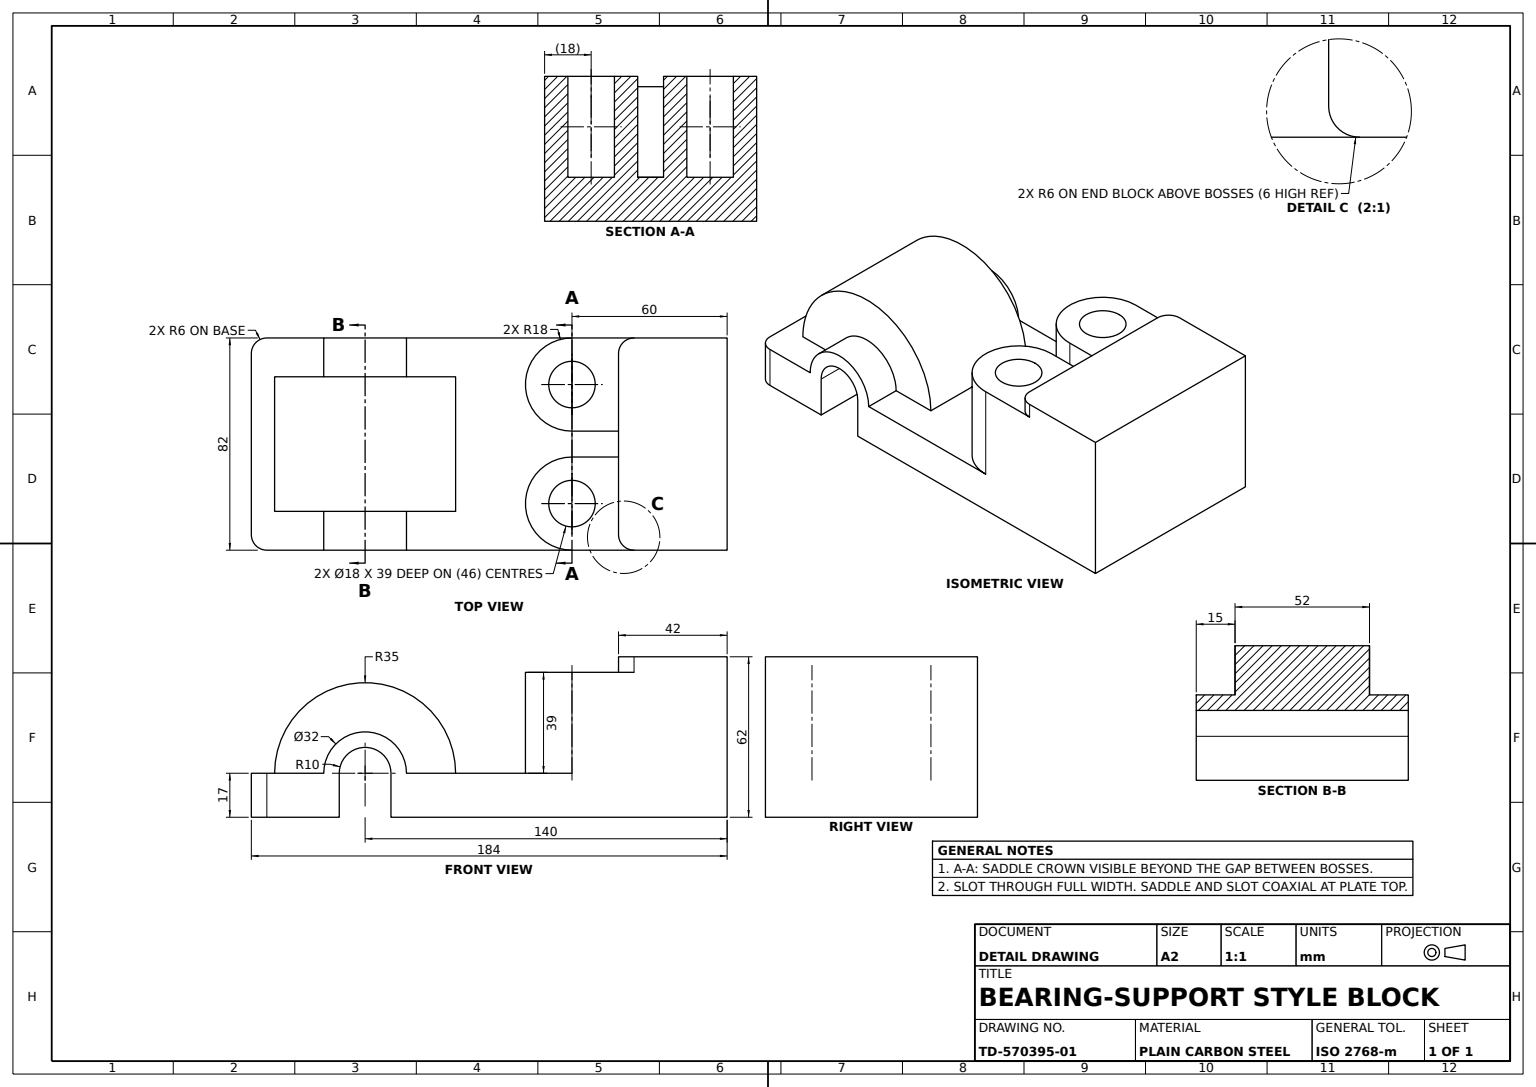
SolidWorks part; units mm, degrees
material "Plain Carbon Steel"
ref_plane "Front Plane" through (0, 0, 0) normal (0, 0, 1) x (1, 0, 0)
ref_plane "Top Plane" through (0, 0, 0) normal (0, 1, 0) x (1, 0, 0)
ref_plane "Right Plane" through (0, 0, 0) normal (1, 0, 0) x (0, 0, -1)
sketch "Base Plate Sketch" plane through (0, 0, 0) normal (0, 1, 0) x (1, 0, 0)
  line L1 (-86, -41) -> (92, -41)
  line L2 (-92, -35) -> (-92, 35)
  line L3 (-86, 41) -> (92, 41)
  line L4 (92, -41) -> (92, 41)
  line L5 (-92, -41) -> (92, 41) construction
  line L6 (-92, 41) -> (92, -41) construction
  arc A0 (-86, -41) -> (-92, -35) centre (-86, -35) cw
  arc A1 (-92, 35) -> (-86, 41) centre (-86, 35) cw
  point P0 (0, 0)
  dimension "D3" = 6
  dimension "D1" = 82
  dimension "D2" = 184
extrude "Base Plate 184x82x17" add sketch "Base Plate Sketch" along normal blind 17
sketch "Bearing Saddle Sketch" plane through (0, 17, 0) normal (0, 1, 0) x (1, 0, 0)
  line L0 (92, 41) -> (-86, 41) construction
  line L1 (92, -41) -> (56, -41)
  line L2 (92, -41) -> (92, 41)
  line L3 (92, 41) -> (56, 41)
  line L4 (50, -35) -> (50, 35)
  arc A0 (56, -41) -> (50, -35) centre (56, -35) cw
  arc A1 (56, 41) -> (50, 35) centre (56, 35) ccw
  point P11 (50, 41)
  dimension "D2" = 6
  dimension "D1" = 42
extrude "Bearing Saddle" add sketch "Bearing Saddle Sketch" along normal blind 45
sketch "Raised Pad Sketch" plane through (0, 0, 41) normal (0, 0, 1) x (1, 0, 0)
  line L0 (-86, 17) -> (56, 17) construction
  line L1 (92, 62) -> (92, 0) construction
  line L2 (-58, 17) -> (-58, 0)
  line L3 (-86, 0) -> (92, 0) construction
  line L4 (-58, 0) -> (-38, 0)
  line L5 (-38, 0) -> (-38, 17)
  arc A0 (-38, 17) -> (-58, 17) centre (-48, 17) ccw
  dimension "D1" = 140
  dimension "D2" = 10
extrude "Raised Pad" add sketch "Raised Pad Sketch" against normal blind 82
sketch "Step Profile Sketch" plane through (0, 0, 41) normal (0, 0, 1) x (1, 0, 0)
  line L0 (-58, 17) -> (-58, 0)
  line L1 (-86, 0) -> (92, 0) construction
  line L2 (-58, 0) -> (-38, 0)
  line L3 (-38, 0) -> (-38, 17)
  line L4 (-86, 17) -> (-64, 17)
  line L5 (-38, 17) -> (-32, 17)
  line L6 (-58, 17) -> (-64, 17)
  arc A0 (-58, 17) -> (-38, 17) centre (-48, 17) cw
  arc A1 (-32, 17) -> (-64, 17) centre (-48, 17) ccw
  line M5 (56, 17) -> (-38, 17)
  arc M6 (-38, 17) -> (-58, 17) centre (-48, 17) ccw
  line M7 (-58, 17) -> (-86, 17)
  dimension "D1" = 10
  dimension "D2" = 32
extrude "Step Profile" add sketch "Step Profile Sketch" against normal blind 82 contours A1 M5 M7 M6
sketch "Slot Cut Sketch" plane through (0, 0, 41) normal (0, 0, 1) x (1, 0, 0)
  line L0 (-58, 17) -> (-58, 0)
  line L1 (-86, 0) -> (92, 0) construction
  line L2 (-58, 0) -> (-38, 0)
  line L3 (-38, 0) -> (-38, 17)
  arc A0 (-38, 17) -> (-58, 17) centre (-48, 17) ccw
  dimension "D1" = 10
extrude "Slot Cut" cut sketch "Slot Cut Sketch" against normal blind 82
sketch "Bolt Bosses Sketch" plane through (0, 17, 0) normal (0, 1, 0) x (1, 0, 0)
  line L0 (32, 41) -> (56, 41)
  line L1 (92, -41) -> (92, 41) construction
  line L2 (32, 5) -> (56, 5)
  line L3 (56, 41) -> (56, 5)
  line L4 (32, -5) -> (56, -5)
  line L5 (56, -5) -> (56, -41)
  line L6 (56, -41) -> (32, -41)
  circle A0 centre (32, 23) radius 9
  circle A1 centre (32, -23) radius 9
  arc A2 (32, 41) -> (32, 5) centre (32, 23) ccw
  arc A3 (32, -5) -> (32, -41) centre (32, -23) ccw
  dimension "D1" = 36
  dimension "D2" = 36
  dimension "D3" = 18
  dimension "D4" = 18
  dimension "D5" = 46
  dimension "D6" = 23
  dimension "D7" = 60
  dimension "D8" = 60
extrude "Bolt Bosses 2x with Holes" add sketch "Bolt Bosses Sketch" along normal blind 39
ref_plane "Plane1" through (0, 0, 0) normal (0, 0, 1) x (1, 0, 0)
sketch "End Block Sketch" plane through (0, 0, 0) normal (0, 0, 1) x (1, 0, 0)
  line L1 (-83, 17) -> (-64, 17)
  line L2 (-32, 17) -> (-13, 17)
  arc A0 (-13, 17) -> (-83, 17) centre (-48, 17) ccw
  arc A2 (-32, 17) -> (-64, 17) centre (-48, 17) ccw construction
  arc A3 (-64, 17) -> (-32, 17) centre (-48, 17) cw
  dimension "D1" = 35
  dimension "D2" = 16
extrude "End Block" add sketch "End Block Sketch" along normal mid plane 52
